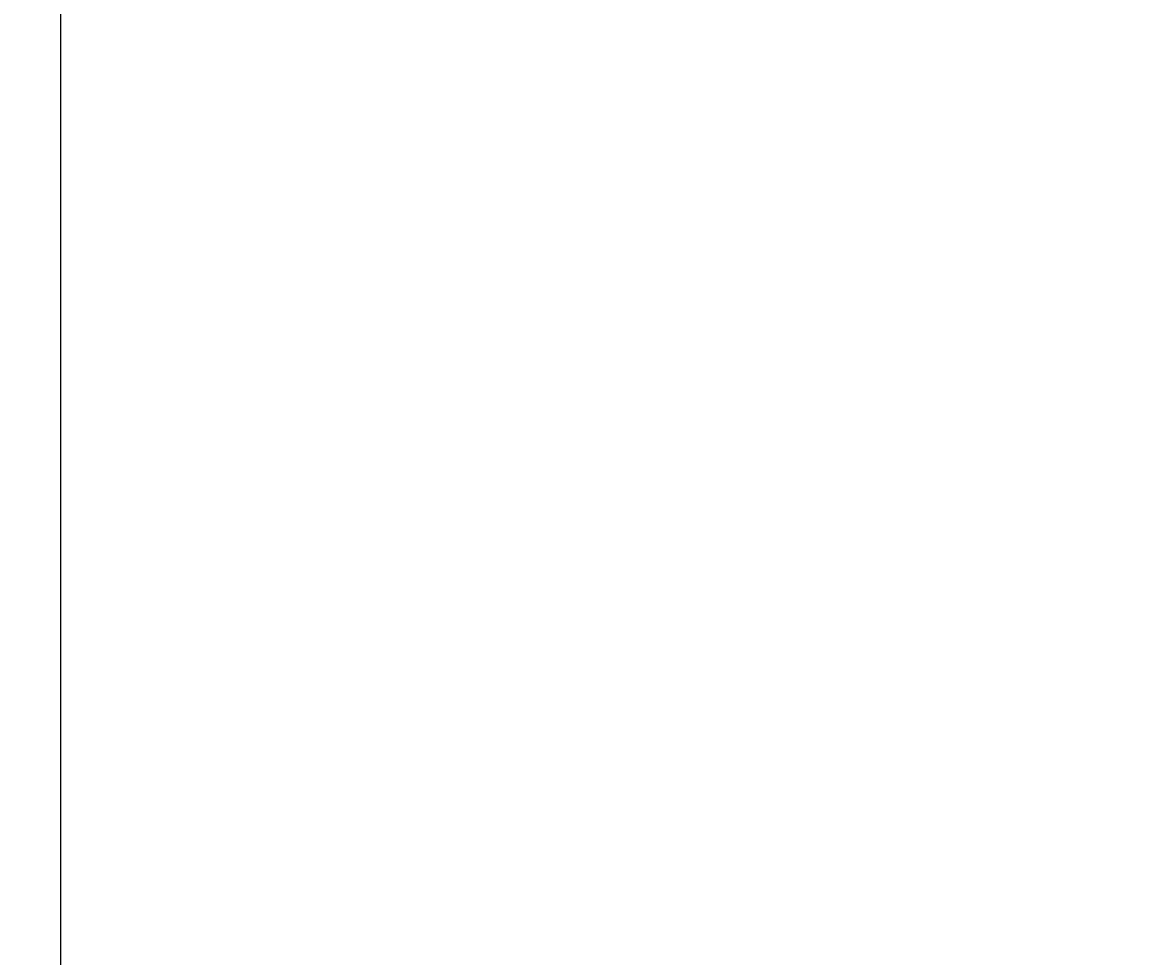
# Model space of a CAD drawing. Units: millimetres. Extents: x 27017497 to 27018854, y 7058029 to 7059154.
# Tile 10 of 91: x 27017560 to 27017605, y 7058200 to 7058238. Entities that reach past the tile are written whole.
import ezdxf

# ---------------------------------------------------------------- set-up
doc = ezdxf.new("R2010")
doc.units = ezdxf.units.MM
doc.layers.add('A-ANNO-DIMS', color=2, linetype='Continuous', lineweight=18)
doc.styles.get("Standard").update_dxf_attribs({"font": 'arial.ttf'})
doc.dimstyles.get("Standard").update_dxf_attribs({"dimtxt": 0.18, "dimasz": 0.18, "dimexe": 0.18, "dimexo": 0.0625, "dimgap": 0.09, "dimtad": 0, "dimtih": 1, "dimtoh": 1, "dimdec": 4, "dimzin": 0, "dimdsep": 46, "dimtxsty": 'Standard', "dimcen": 0.09, "dimadec": 0, "dimazin": 0, "dimtfac": 1, "dimtdec": 4, "dimtofl": 0, "dimtmove": 0, "dimatfit": 3, "dimfxl": 1, "dimtolj": 1, "dimtzin": 0, "dimarcsym": 0})

# ---------------------------------------------------------------- blocks, each defined once
blk = doc.blocks.new('*D47')
at = {"layer": 'A-ANNO-DIMS', "color": 0, "lineweight": -2, "transparency": 16777216}
for p, q in [((27017561.166, 7058294.35), (27017561.166, 7058028.6)), ((27018790.606, 7058294.35), (27018790.606, 7058028.6)), ((27017561.346, 7058028.78), (27018175.431, 7058028.78)), ((27018790.426, 7058028.78), (27018176.341, 7058028.78))]:
    blk.add_line(p, q, dxfattribs=at)
at = {"layer": 'A-ANNO-DIMS', "color": 0, "transparency": 16777216}
for points in [[(27017561.346, 7058028.81), (27017561.346, 7058028.75), (27017561.166, 7058028.78)], [(27018790.426, 7058028.81), (27018790.426, 7058028.75), (27018790.606, 7058028.78)]]:
    blk.add_solid(points, dxfattribs=at)
at = {"layer": 'Defpoints', "color": 0, "transparency": 16777216}
for p in [(27017561.166, 7058294.412), (27018790.606, 7058294.412), (27018790.606, 7058028.78)]:
    blk.add_point(p, dxfattribs=at)
at = {"layer": 'A-ANNO-DIMS', "color": 0, "transparency": 16777216, "insert": (27018175.886, 7058028.78), "char_height": 0.18, "attachment_point": 5}
blk.add_mtext('\\A1;1229.4', dxfattribs=at)
blk = doc.blocks.new('*D48')
at = {"layer": 'A-ANNO-DIMS', "color": 0, "lineweight": -2, "transparency": 16777216}
for p, q in [((27018463.498, 7058622.912), (27017497.536, 7058622.912)), ((27017497.716, 7058622.732), (27017497.716, 7058357.753)), ((27017497.716, 7058092.41), (27017497.716, 7058357.389)), ((27018555.129, 7058092.23), (27017497.536, 7058092.23))]:
    blk.add_line(p, q, dxfattribs=at)
at = {"layer": 'A-ANNO-DIMS', "color": 0, "transparency": 16777216}
for points in [[(27017497.686, 7058622.732), (27017497.746, 7058622.732), (27017497.716, 7058622.912)], [(27017497.686, 7058092.41), (27017497.746, 7058092.41), (27017497.716, 7058092.23)]]:
    blk.add_solid(points, dxfattribs=at)
at = {"layer": 'Defpoints', "color": 0, "transparency": 16777216}
for p in [(27018463.561, 7058622.912), (27017497.716, 7058092.23), (27018555.192, 7058092.23)]:
    blk.add_point(p, dxfattribs=at)
at = {"layer": 'A-ANNO-DIMS', "color": 0, "transparency": 16777216, "insert": (27017497.716, 7058357.571), "char_height": 0.18, "attachment_point": 5}
blk.add_mtext('\\A1;530.7', dxfattribs=at)

msp = doc.modelspace()

# ---------------------------------------------------------------- dimensions: what is measured, and where the dimension line sits
at = {"layer": 'A-ANNO-DIMS'}
dim = msp.add_linear_dim(base=(27017497.716, 7058092.23), p1=(27018463.561, 7058622.912), p2=(27018555.192, 7058092.23), angle=90, dimstyle='Standard', override={"dimdec": 1, "dimlfac": 1, "dimrnd": 0, "dimzin": 0, "dimdsep": 46, "dimlunit": 2}, dxfattribs=at)
dim.commit()
dim.dimension.update_dxf_attribs({"geometry": '*D48', "text_midpoint": (27017497.716, 7058357.571)})
dim = msp.add_linear_dim(base=(27018790.606, 7058028.78), p1=(27017561.166, 7058294.412), p2=(27018790.606, 7058294.412), dimstyle='Standard', override={"dimdec": 1, "dimlfac": 1, "dimrnd": 0, "dimzin": 0, "dimdsep": 46, "dimlunit": 2}, dxfattribs=at)
dim.commit()
dim.dimension.update_dxf_attribs({"geometry": '*D47', "text_midpoint": (27018175.886, 7058028.78)})

doc.saveas('drawing.dxf')
